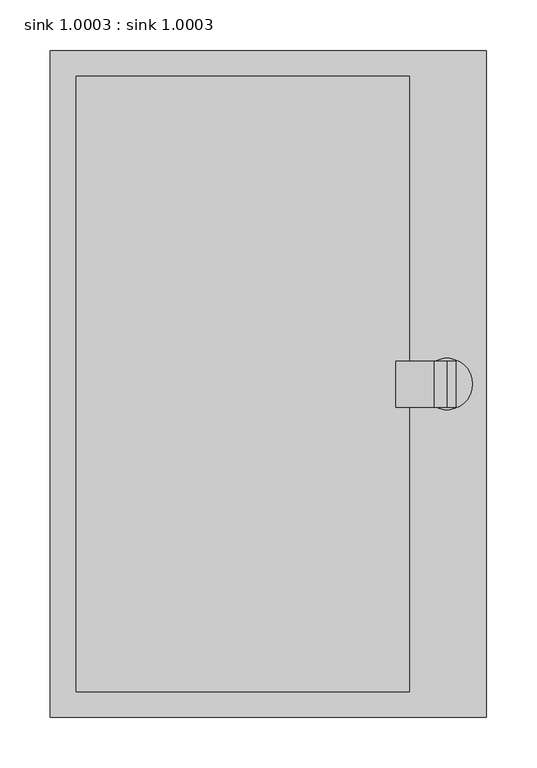
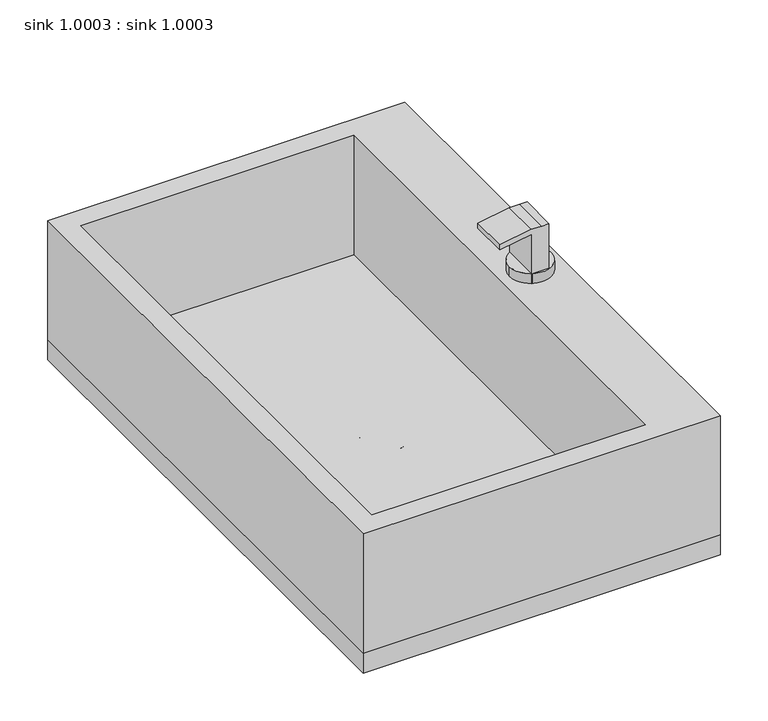
"""IFC4 building model written with IfcOpenShell, lengths in millimetres: flow terminal geometry, sink 1.0003 : sink 1.0003."""

from ifc_helpers import new_model, si_unit, point, frame, frame_2d, origin, origin_with_axes, place, context, project, spatial, polyline, circle_curve, trimmed, segment, composite_curve, outline, extrude, source, transform, mapped, element, save


def sink_1_0003_sink_1_0003_9aba45dc(model_context):
    return source(origin(), model_context, "Body", "SweptSolid", [
        extrude(outline(polyline([(215.9, 330.2), (215.9, -330.2), (-215.9, -330.2), (-215.9, 330.2), (215.9, 330.2)]), holes=[polyline([(139.7, -304.8), (139.7, 304.8), (-190.5, 304.8), (-190.5, -304.8), (139.7, -304.8)])]), origin_with_axes(), (0.0, 0.0, 1.0), 152.4),
        extrude(outline(polyline([(215.9, 330.2), (215.9, -330.2), (-215.9, -330.2), (-215.9, 330.2), (215.9, 330.2)])), frame((0.0, 0.0, -25.4), z_axis=(0.0, 0.0, 1.0), x_axis=(1.0, 0.0, 0.0)), (0.0, 0.0, 1.0), 25.4),
        extrude(outline(composite_curve([segment(trimmed(circle_curve(frame_2d((176.9682898, 0.0)), 25.4), [point((151.5682898, 0.0))], [point((202.3682898, 0.0))], False, "CARTESIAN"), True, "CONTINUOUS"), segment(trimmed(circle_curve(frame_2d((176.9682898, 0.0)), 25.4), [point((202.3682898, 0.0))], [point((151.5682898, 0.0))], False, "CARTESIAN"), True, "CONTINUOUS")], self_intersect=False)), frame((0.0, 0.0, 152.4), z_axis=(0.0, 0.0, 1.0), x_axis=(1.0, 0.0, 0.0)), (0.0, 0.0, 1.0), 12.7),
        extrude(outline(polyline([(215.7984477, 165.1), (152.4, 165.1), (152.4, 185.9356273), (222.25, 185.9356273), (222.25, 177.2345539), (222.25, 164.5345539), (216.09293, 126.4345539), (209.55, 126.4345539), (215.7984477, 165.1)])), frame((0.0, -23.2093179, 0.0), z_axis=(0.0, 1.0, 0.0), x_axis=(0.0, 0.0, 1.0)), (0.0, 0.0, 1.0), 45.6225728),
        extrude(outline(composite_curve([segment(trimmed(circle_curve(frame_2d((139.7, 0.0)), 6.35), [point((133.35, 0.0))], [point((146.05, 0.0))], False, "CARTESIAN"), True, "CONTINUOUS"), segment(trimmed(circle_curve(frame_2d((139.7, 0.0)), 6.35), [point((146.05, 0.0))], [point((133.35, 0.0))], False, "CARTESIAN"), True, "CONTINUOUS")], self_intersect=False)), frame((0.0, 0.0, 209.55), z_axis=(0.0, 0.0, 1.0), x_axis=(1.0, 0.0, 0.0)), (0.0, 0.0, 1.0), 4.2003995),
        extrude(outline(composite_curve([segment(trimmed(circle_curve(frame_2d((-1.2158564, -1.9862296)), 25.4), [point((-26.6158564, -1.9862296))], [point((24.1841436, -1.9862296))], False, "CARTESIAN"), True, "CONTINUOUS"), segment(trimmed(circle_curve(frame_2d((-1.2158564, -1.9862296)), 25.4), [point((24.1841436, -1.9862296))], [point((-26.6158564, -1.9862296))], False, "CARTESIAN"), True, "CONTINUOUS")], self_intersect=False)), frame((0.0, 0.0, -25.4), z_axis=(0.0, 0.0, 1.0), x_axis=(1.0, 0.0, 0.0)), (0.0, 0.0, 1.0), 25.4),
    ])


if __name__ == "__main__":
    model = new_model("IFC4")
    model_context = context("Model", 3, world=origin())
    ifc_project = project(units=[si_unit("LENGTHUNIT", "METRE", prefix="MILLI")], contexts=[model_context])
    site = spatial("IfcSite", under=ifc_project)
    building = spatial("IfcBuilding", under=site)
    placement = place(None, origin())
    sink_1_0003_sink_1_0003_shape = sink_1_0003_sink_1_0003_9aba45dc(model_context)
    element("IfcFlowTerminal", 1, ObjectType="sink 1.0003 : sink 1.0003", at=placement, inside=building, context=model_context, shape_type="MappedRepresentation", body=[
        mapped(sink_1_0003_sink_1_0003_shape, transform((0.0, 0.0, 0.0), x_axis=(1.0, 0.0, 0.0), y_axis=(0.0, 1.0, 0.0), z_axis=(0.0, 0.0, 1.0))),
    ])
    save(model, "model.ifc")

# Revit data of these elements
# Type "sink 1.0003 : sink 1.0003"
#   Default Elevation = 0
# Element 1 (IfcFlowTerminal, "sink 1.0003 : sink 1.0003")
#   Materials on its faces: "steel", "sink"
# Materials
#   "steel": class "Generic", colour RGB 244 245 246, transparency 0, Cost = 0
#   "sink": class "Generic", colour RGB 120 120 120, transparency 0, Cost = 0
